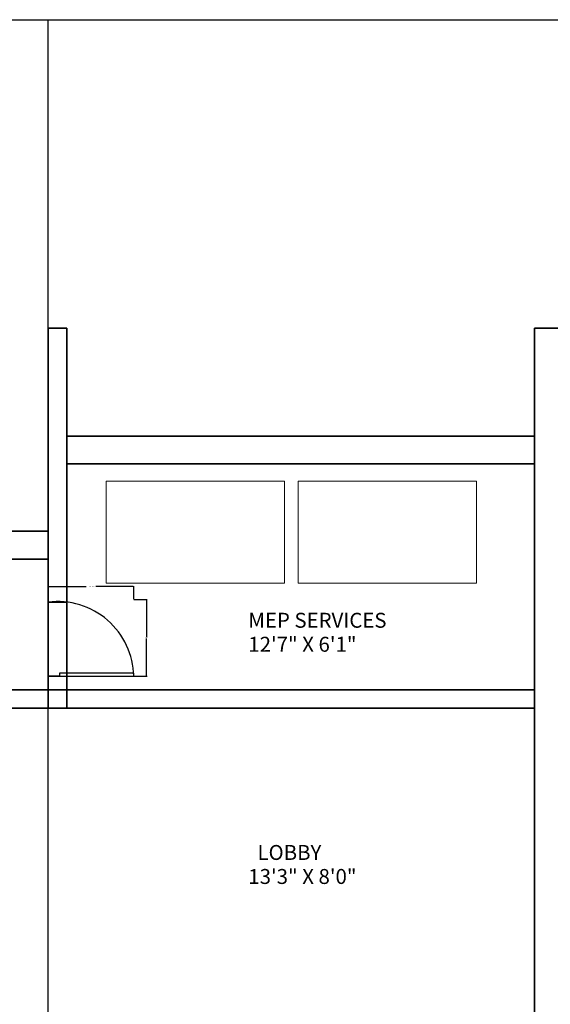
# Model space of a CAD drawing. Units: inches. Extents: x -61 to 1599, y -1316 to 257.
# Tile 200 of 204: x 826 to 998, y -61 to 257. Entities that reach past the tile are written whole.
import ezdxf

# ---------------------------------------------------------------- set-up
doc = ezdxf.new("R2010")
doc.units = ezdxf.units.IN
doc.header["$MEASUREMENT"] = 0
doc.linetypes.add('ACAD_ISO02W100', pattern=[15, 12, -3])
for name, color, linetype, lineweight in [('A-ANNO-DIMS', 2, 'Continuous', 18), ('A-AREA-IDEN', 1, 'Continuous', 18), ('A-EQPM', 9, 'Continuous', 18), ('A-WALL-JAMB', 4, 'ACAD_ISO02W100', 25), ('DOORS', 2, 'Continuous', 25), ('WALLS', 4, 'Continuous', 35)]:
    doc.layers.add(name, color=color, linetype=linetype, lineweight=lineweight)
doc.styles.get("Standard").update_dxf_attribs({"font": 'arial.ttf'})
doc.dimstyles.get("Standard").update_dxf_attribs({"dimtxt": 0.18, "dimasz": 0.18, "dimexe": 0.18, "dimexo": 0.0625, "dimgap": 0.09, "dimtad": 0, "dimtih": 1, "dimtoh": 1, "dimdec": 0, "dimzin": 0, "dimdsep": 46, "dimlunit": 3, "dimtxsty": 'Standard', "dimcen": 0.09, "dimadec": 0, "dimazin": 0, "dimtfac": 1, "dimtdec": 0, "dimtofl": 0, "dimtmove": 0, "dimatfit": 3, "dimfxl": 1, "dimtolj": 1, "dimtzin": 0, "dimarcsym": 0})

# ---------------------------------------------------------------- blocks, each defined once
blk = doc.blocks.new('DOOR-SWING-24')
blk.add_line((0, 0), (0, 3.6))
blk.add_lwpolyline([(0, 0), (0, -24), (1.05, -24), (1.05, 0)], close=True)
blk.add_arc((-0.44, 0.62), 24.62, 271.0259, 6.9559)
blk = doc.blocks.new('*D610')
at = {"layer": 'A-ANNO-DIMS', "color": 0, "lineweight": -2, "transparency": 16777216}
for p, q in [((835.7, 70.09), (835.7, 74.35)), ((835.88, 74.17), (847.98, 74.17)), ((863.12, 74.17), (851.03, 74.17)), ((863.3, 70.09), (863.3, 74.35))]:
    blk.add_line(p, q, dxfattribs=at)
at = {"layer": 'A-ANNO-DIMS', "color": 0, "transparency": 16777216}
for points in [[(835.88, 74.2), (835.88, 74.14), (835.7, 74.17)], [(863.12, 74.2), (863.12, 74.14), (863.3, 74.17)]]:
    blk.add_solid(points, dxfattribs=at)
at = {"layer": 'DEFPOINTS', "color": 0, "transparency": 16777216}
for p in [(835.7, 74.17), (835.7, 70.03), (863.3, 70.03)]:
    blk.add_point(p, dxfattribs=at)
at = {"layer": 'A-ANNO-DIMS', "color": 0, "transparency": 16777216, "insert": (849.5, 74.17), "char_height": 0.18, "attachment_point": 5}
blk.add_mtext('\\A1;SERVICE DOOR 28 TYP.', dxfattribs=at)
blk = doc.blocks.new('*D611')
at = {"layer": 'A-ANNO-DIMS', "color": 0, "lineweight": -2, "transparency": 16777216}
for p, q in [((863.37, 70.03), (867.62, 70.03)), ((867.44, 69.85), (867.44, 57.79)), ((867.44, 45.37), (867.44, 57.43)), ((863.37, 45.19), (867.62, 45.19))]:
    blk.add_line(p, q, dxfattribs=at)
at = {"layer": 'A-ANNO-DIMS', "color": 0, "transparency": 16777216}
for points in [[(867.41, 69.85), (867.47, 69.85), (867.44, 70.03)], [(867.41, 45.37), (867.47, 45.37), (867.44, 45.19)]]:
    blk.add_solid(points, dxfattribs=at)
at = {"layer": 'DEFPOINTS', "color": 0, "transparency": 16777216}
for p in [(863.3, 70.03), (867.44, 70.03), (863.3, 45.19)]:
    blk.add_point(p, dxfattribs=at)
at = {"layer": 'A-ANNO-DIMS', "color": 0, "transparency": 16777216, "insert": (867.44, 57.61), "char_height": 0.18, "attachment_point": 5}
blk.add_mtext('\\A1;25 TYP.', dxfattribs=at)
blk = doc.blocks.new('*D686')
at = {"layer": 'A-ANNO-DIMS', "color": 0, "lineweight": -2, "transparency": 16777216}
for p, q in [((14.7, 157.74), (14.7, 257.46)), ((14.88, 257.28), (768.35, 257.28)), ((1522.52, 257.28), (769.05, 257.28)), ((1522.7, 157.74), (1522.7, 257.46))]:
    blk.add_line(p, q, dxfattribs=at)
at = {"layer": 'A-ANNO-DIMS', "color": 0, "transparency": 16777216}
for points in [[(14.88, 257.31), (14.88, 257.25), (14.7, 257.28)], [(1522.52, 257.31), (1522.52, 257.25), (1522.7, 257.28)]]:
    blk.add_solid(points, dxfattribs=at)
at = {"layer": 'DEFPOINTS', "color": 0, "transparency": 16777216}
for p in [(1522.7, 257.28), (14.7, 157.68), (1522.7, 157.68)]:
    blk.add_point(p, dxfattribs=at)
at = {"layer": 'A-ANNO-DIMS', "color": 0, "transparency": 16777216, "insert": (768.7, 257.28), "char_height": 0.18, "attachment_point": 5}
blk.add_mtext('\\A1;1508', dxfattribs=at)
blk = doc.blocks.new('*D697')
at = {"layer": 'A-ANNO-DIMS', "color": 0, "lineweight": -2, "transparency": 16777216}
for p, q in [((644.7, -561.11), (644.7, 257.46)), ((644.88, 257.28), (739.94, 257.28)), ((835.52, 257.28), (740.47, 257.28)), ((835.7, -563.19), (835.7, 257.46))]:
    blk.add_line(p, q, dxfattribs=at)
at = {"layer": 'A-ANNO-DIMS', "color": 0, "transparency": 16777216}
for points in [[(644.88, 257.31), (644.88, 257.25), (644.7, 257.28)], [(835.52, 257.31), (835.52, 257.25), (835.7, 257.28)]]:
    blk.add_solid(points, dxfattribs=at)
at = {"layer": 'DEFPOINTS', "color": 0, "transparency": 16777216}
for p in [(835.7, 257.28), (644.7, -561.17), (835.7, -563.25)]:
    blk.add_point(p, dxfattribs=at)
at = {"layer": 'A-ANNO-DIMS', "color": 0, "transparency": 16777216, "insert": (740.2, 257.28), "char_height": 0.18, "attachment_point": 5}
blk.add_mtext('\\A1;191', dxfattribs=at)

msp = doc.modelspace()

# ---------------------------------------------------------------- linework, layer by layer
at = {"layer": 'A-EQPM'}
for points in [[(912.0479, 75.2853), (854.4503, 75.2853), (854.4503, 108.2545), (912.0479, 108.2545)], [(974.0014, 75.2853), (916.4038, 75.2853), (916.4038, 108.2545), (974.0014, 108.2545)]]:
    msp.add_lwpolyline(points, close=True, dxfattribs=at)
at = {"layer": 'A-WALL-JAMB'}
for p, q in [((835.7028, 69.188), (841.7028, 69.1836)), ((835.7028, 45.188), (841.7028, 45.188))]:
    msp.add_line(p, q, dxfattribs=at)
at = {"layer": 'WALLS'}
for p, q in [((835.7028, 157.6771), (835.7028, 34.831)), ((835.7028, 157.6771), (841.7028, 157.6771)), ((841.7028, 157.6771), (841.7028, 34.831)), ((992.7028, 157.6771), (992.7028, 34.831)), ((992.7028, 157.6771), (992.7028, -441.3229)), ((1522.7028, 157.6771), (992.7028, 157.6771)), ((841.7028, 122.831), (992.7028, 122.831)), ((841.7028, 113.831), (992.7028, 113.831)), ((685.7028, 92.0619), (835.7028, 92.0619)), ((685.7028, 83.0619), (835.7028, 83.0619)), ((544.7028, 40.831), (992.7028, 40.831)), ((544.7028, 34.831), (992.7028, 34.831)), ((992.7028, -61.169), (992.7028, 34.831))]:
    msp.add_line(p, q, dxfattribs=at)

# ---------------------------------------------------------------- block references
at = {"layer": 'DOORS', "rotation": 90.00000000000036}
msp.add_blockref('DOOR-SWING-24', (839.3028, 45.188), dxfattribs=at)

# ---------------------------------------------------------------- texts
at = {"layer": 'A-AREA-IDEN'}
for s, height, p in [('MEP SERVICES', 4.832098, (900.3213, 60.8788)), ('12\'7" X 6\'1"', 4.832098, (900.3213, 53.1165)), ('  LOBBY', 4.8321, (900.3213, -14.1883)), ('13\'3" X 8\'0"', 4.832098, (900.3213, -21.9506))]:
    msp.add_text(s, height=height, dxfattribs=at).set_placement(p)

# ---------------------------------------------------------------- dimensions: what is measured, and where the dimension line sits
at = {"layer": 'A-ANNO-DIMS'}
for base, p1, p2, picture, middle in [((1522.7028, 257.2771), (14.7028, 157.6771), (1522.7028, 157.6771), '*D686', (768.7028, 257.2771)), ((835.7028, 257.2771), (644.7028, -561.169), (835.7028, -563.2524), '*D697', (740.2028, 257.2771))]:
    dim = msp.add_linear_dim(base=base, p1=p1, p2=p2, dimstyle='Standard', override={"dimdec": 0, "dimlfac": 1, "dimrnd": 0, "dimzin": 0, "dimdsep": 46, "dimlunit": 2}, dxfattribs=at)
    dim.commit()
    dim.dimension.update_dxf_attribs({"geometry": picture, "text_midpoint": middle})
for base, p1, p2, angle, text, picture, middle in [((835.7028, 74.1725), (863.3028, 70.0325), (835.7028, 70.0325), 180, 'SERVICE DOOR <> TYP.', '*D610', (849.5028, 74.1725)), ((867.4428, 70.0325), (863.3028, 45.188), (863.3028, 70.0325), 90, '<> TYP.', '*D611', (867.4428, 57.6102))]:
    dim = msp.add_linear_dim(base=base, p1=p1, p2=p2, angle=angle, text=text, dimstyle='Standard', override={"dimdec": 0, "dimlfac": 1, "dimrnd": 0, "dimzin": 0, "dimdsep": 46, "dimlunit": 2}, dxfattribs=at)
    dim.commit()
    dim.dimension.update_dxf_attribs({"geometry": picture, "text_midpoint": middle})

doc.saveas('drawing.dxf')
